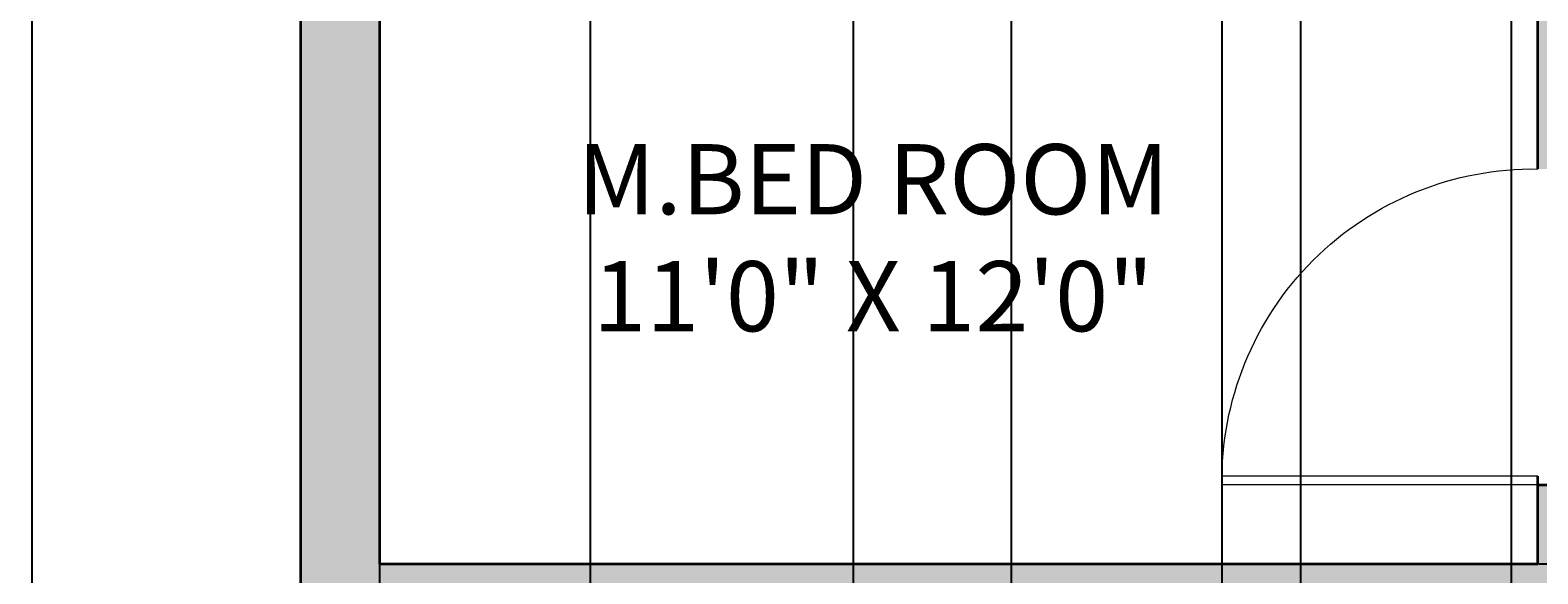
# Model space of a CAD drawing. Units: inches. Extents: x 1567 to 1964, y 1813 to 2447.
# Tile 13 of 28: x 1567 to 1738, y 2262 to 2324. Entities that reach past the tile are written whole.
import ezdxf

# ---------------------------------------------------------------- set-up
doc = ezdxf.new("R2010")
doc.units = ezdxf.units.IN
for name, color, linetype, lineweight in [('A-ANNO-DIMS', 2, 'Continuous', 18), ('A-AREA-IDEN', 7, 'Continuous', 18), ('A-DOOR', 4, 'Continuous', 18), ('A-WALL', 7, 'Continuous', 35)]:
    doc.layers.add(name, color=color, linetype=linetype, lineweight=lineweight)
doc.layers.add('A-WALL-PATT', color=251, linetype='Continuous', lineweight=13, true_color=0x636466)
doc.styles.get("Standard").update_dxf_attribs({"font": 'arial.ttf'})
doc.dimstyles.get("Standard").update_dxf_attribs({"dimtxt": 0.18, "dimasz": 0.18, "dimexe": 0.18, "dimexo": 0.0625, "dimgap": 0.09, "dimtad": 0, "dimtih": 1, "dimtoh": 1, "dimdec": 4, "dimzin": 0, "dimdsep": 46, "dimtxsty": 'Standard', "dimcen": 0.09, "dimadec": 0, "dimazin": 0, "dimtfac": 1, "dimtdec": 4, "dimtofl": 0, "dimtmove": 0, "dimatfit": 3, "dimfxl": 1, "dimtolj": 1, "dimtzin": 0, "dimarcsym": 0})

# ---------------------------------------------------------------- blocks, each defined once
blk = doc.blocks.new('DOOR-SWING-36IN')
for p, q in [((0, 36), (0, 0)), ((1, 36), (1, 0))]:
    blk.add_line(p, q)
blk.add_arc((0.5, 35.5), 35.5, 269.1931, 0.8069)
blk = doc.blocks.new('*D41')
at = {"layer": 'A-ANNO-DIMS', "color": 0, "lineweight": -2, "transparency": 16777216}
for p, q in [((1597.37, 2416.29), (1566.6, 2416.29)), ((1566.78, 2416.11), (1566.78, 2160.47)), ((1566.78, 1904.47), (1566.78, 2160.11)), ((1601.37, 1904.29), (1566.6, 1904.29))]:
    blk.add_line(p, q, dxfattribs=at)
at = {"layer": 'A-ANNO-DIMS', "color": 0, "transparency": 16777216}
for points in [[(1566.75, 2416.11), (1566.81, 2416.11), (1566.78, 2416.29)], [(1566.75, 1904.47), (1566.81, 1904.47), (1566.78, 1904.29)]]:
    blk.add_solid(points, dxfattribs=at)
at = {"layer": 'Defpoints', "color": 0, "transparency": 16777216}
for p in [(1566.78, 2416.29), (1597.43, 2416.29), (1601.43, 1904.29)]:
    blk.add_point(p, dxfattribs=at)
at = {"layer": 'A-ANNO-DIMS', "color": 0, "transparency": 16777216, "insert": (1566.78, 2160.29), "char_height": 0.18, "attachment_point": 5}
blk.add_mtext('\\A1;512', dxfattribs=at)
blk = doc.blocks.new('*D53')
at = {"layer": 'A-ANNO-DIMS', "color": 0, "lineweight": -2, "transparency": 16777216}
for p, q in [((1606.43, 1913.35), (1606.43, 2447.12)), ((1606.61, 2446.94), (1618.21, 2446.94)), ((1630.25, 2446.94), (1618.65, 2446.94)), ((1630.43, 1913.35), (1630.43, 2447.12))]:
    blk.add_line(p, q, dxfattribs=at)
at = {"layer": 'A-ANNO-DIMS', "color": 0, "transparency": 16777216}
for points in [[(1606.61, 2446.97), (1606.61, 2446.91), (1606.43, 2446.94)], [(1630.25, 2446.97), (1630.25, 2446.91), (1630.43, 2446.94)]]:
    blk.add_solid(points, dxfattribs=at)
at = {"layer": 'Defpoints', "color": 0, "transparency": 16777216}
for p in [(1630.43, 2446.94), (1606.43, 1913.29), (1630.43, 1913.29)]:
    blk.add_point(p, dxfattribs=at)
at = {"layer": 'A-ANNO-DIMS', "color": 0, "transparency": 16777216, "insert": (1618.43, 2446.94), "char_height": 0.18, "attachment_point": 5}
blk.add_mtext('\\A1;24', dxfattribs=at)
blk = doc.blocks.new('*D54')
at = {"layer": 'A-ANNO-DIMS', "color": 0, "lineweight": -2, "transparency": 16777216}
for p, q in [((1711.43, 1964.35), (1711.43, 2447.12)), ((1711.61, 2446.94), (1753.21, 2446.94)), ((1795.25, 2446.94), (1753.65, 2446.94)), ((1795.43, 1964.35), (1795.43, 2447.12))]:
    blk.add_line(p, q, dxfattribs=at)
at = {"layer": 'A-ANNO-DIMS', "color": 0, "transparency": 16777216}
for points in [[(1711.61, 2446.97), (1711.61, 2446.91), (1711.43, 2446.94)], [(1795.25, 2446.97), (1795.25, 2446.91), (1795.43, 2446.94)]]:
    blk.add_solid(points, dxfattribs=at)
at = {"layer": 'Defpoints', "color": 0, "transparency": 16777216}
for p in [(1795.43, 2446.94), (1711.43, 1964.29), (1795.43, 1964.29)]:
    blk.add_point(p, dxfattribs=at)
at = {"layer": 'A-ANNO-DIMS', "color": 0, "transparency": 16777216, "insert": (1753.43, 2446.94), "char_height": 0.18, "attachment_point": 5}
blk.add_mtext('\\A1;84', dxfattribs=at)
blk = doc.blocks.new('*D56')
at = {"layer": 'A-ANNO-DIMS', "color": 0, "lineweight": -2, "transparency": 16777216}
for p, q in [((1606.43, 2127.35), (1606.43, 2447.12)), ((1606.61, 2446.94), (1618.21, 2446.94)), ((1630.25, 2446.94), (1618.65, 2446.94)), ((1630.43, 2127.35), (1630.43, 2447.12))]:
    blk.add_line(p, q, dxfattribs=at)
at = {"layer": 'A-ANNO-DIMS', "color": 0, "transparency": 16777216}
for points in [[(1606.61, 2446.97), (1606.61, 2446.91), (1606.43, 2446.94)], [(1630.25, 2446.97), (1630.25, 2446.91), (1630.43, 2446.94)]]:
    blk.add_solid(points, dxfattribs=at)
at = {"layer": 'Defpoints', "color": 0, "transparency": 16777216}
for p in [(1630.43, 2446.94), (1606.43, 2127.29), (1630.43, 2127.29)]:
    blk.add_point(p, dxfattribs=at)
at = {"layer": 'A-ANNO-DIMS', "color": 0, "transparency": 16777216, "insert": (1618.43, 2446.94), "char_height": 0.18, "attachment_point": 5}
blk.add_mtext('\\A1;24', dxfattribs=at)
blk = doc.blocks.new('*D57')
at = {"layer": 'A-ANNO-DIMS', "color": 0, "lineweight": -2, "transparency": 16777216}
for p, q in [((1630.43, 2127.35), (1630.43, 2447.12)), ((1630.61, 2446.94), (1654.21, 2446.94)), ((1678.25, 2446.94), (1654.65, 2446.94)), ((1678.43, 2127.35), (1678.43, 2447.12))]:
    blk.add_line(p, q, dxfattribs=at)
at = {"layer": 'A-ANNO-DIMS', "color": 0, "transparency": 16777216}
for points in [[(1630.61, 2446.97), (1630.61, 2446.91), (1630.43, 2446.94)], [(1678.25, 2446.97), (1678.25, 2446.91), (1678.43, 2446.94)]]:
    blk.add_solid(points, dxfattribs=at)
at = {"layer": 'Defpoints', "color": 0, "transparency": 16777216}
for p in [(1678.43, 2446.94), (1630.43, 2127.29), (1678.43, 2127.29)]:
    blk.add_point(p, dxfattribs=at)
at = {"layer": 'A-ANNO-DIMS', "color": 0, "transparency": 16777216, "insert": (1654.43, 2446.94), "char_height": 0.18, "attachment_point": 5}
blk.add_mtext('\\A1;48', dxfattribs=at)
blk = doc.blocks.new('*D60')
at = {"layer": 'A-ANNO-DIMS', "color": 0, "lineweight": -2, "transparency": 16777216}
for p, q in [((1660.43, 2063.35), (1660.43, 2447.12)), ((1660.61, 2446.94), (1681.21, 2446.94)), ((1702.25, 2446.94), (1681.65, 2446.94)), ((1702.43, 2063.35), (1702.43, 2447.12))]:
    blk.add_line(p, q, dxfattribs=at)
at = {"layer": 'A-ANNO-DIMS', "color": 0, "transparency": 16777216}
for points in [[(1660.61, 2446.97), (1660.61, 2446.91), (1660.43, 2446.94)], [(1702.25, 2446.97), (1702.25, 2446.91), (1702.43, 2446.94)]]:
    blk.add_solid(points, dxfattribs=at)
at = {"layer": 'Defpoints', "color": 0, "transparency": 16777216}
for p in [(1660.43, 2446.94), (1660.43, 2063.29), (1702.43, 2063.29)]:
    blk.add_point(p, dxfattribs=at)
at = {"layer": 'A-ANNO-DIMS', "color": 0, "transparency": 16777216, "insert": (1681.43, 2446.94), "char_height": 0.18, "attachment_point": 5}
blk.add_mtext('\\A1;42', dxfattribs=at)
blk = doc.blocks.new('*D63')
at = {"layer": 'A-ANNO-DIMS', "color": 0, "lineweight": -2, "transparency": 16777216}
for p, q in [((1735.43, 1988.35), (1735.43, 2447.12)), ((1735.61, 2446.94), (1753.21, 2446.94)), ((1771.25, 2446.94), (1753.65, 2446.94)), ((1771.43, 1988.35), (1771.43, 2447.12))]:
    blk.add_line(p, q, dxfattribs=at)
at = {"layer": 'A-ANNO-DIMS', "color": 0, "transparency": 16777216}
for points in [[(1735.61, 2446.97), (1735.61, 2446.91), (1735.43, 2446.94)], [(1771.25, 2446.97), (1771.25, 2446.91), (1771.43, 2446.94)]]:
    blk.add_solid(points, dxfattribs=at)
at = {"layer": 'Defpoints', "color": 0, "transparency": 16777216}
for p in [(1771.43, 2446.94), (1735.43, 1988.29), (1771.43, 1988.29)]:
    blk.add_point(p, dxfattribs=at)
at = {"layer": 'A-ANNO-DIMS', "color": 0, "transparency": 16777216, "insert": (1753.43, 2446.94), "char_height": 0.18, "attachment_point": 5}
blk.add_mtext('\\A1;36', dxfattribs=at)
blk = doc.blocks.new('*D64')
at = {"layer": 'A-ANNO-DIMS', "color": 0, "lineweight": -2, "transparency": 16777216}
for p, q in [((1711.43, 2055.85), (1711.43, 2447.12)), ((1711.61, 2446.94), (1723.21, 2446.94)), ((1735.25, 2446.94), (1723.65, 2446.94)), ((1735.43, 2055.85), (1735.43, 2447.12))]:
    blk.add_line(p, q, dxfattribs=at)
at = {"layer": 'A-ANNO-DIMS', "color": 0, "transparency": 16777216}
for points in [[(1711.61, 2446.97), (1711.61, 2446.91), (1711.43, 2446.94)], [(1735.25, 2446.97), (1735.25, 2446.91), (1735.43, 2446.94)]]:
    blk.add_solid(points, dxfattribs=at)
at = {"layer": 'Defpoints', "color": 0, "transparency": 16777216}
for p in [(1735.43, 2446.94), (1711.43, 2055.79), (1735.43, 2055.79)]:
    blk.add_point(p, dxfattribs=at)
at = {"layer": 'A-ANNO-DIMS', "color": 0, "transparency": 16777216, "insert": (1723.43, 2446.94), "char_height": 0.18, "attachment_point": 5}
blk.add_mtext('\\A1;24', dxfattribs=at)
blk = doc.blocks.new('*D68')
at = {"layer": 'A-ANNO-DIMS', "color": 0, "lineweight": -2, "transparency": 16777216}
for p, q in [((1738.49, 2272.29), (1769.26, 2272.29)), ((1769.08, 2272.11), (1769.08, 2267.97)), ((1769.08, 2263.47), (1769.08, 2267.61)), ((1738.49, 2263.29), (1769.26, 2263.29))]:
    blk.add_line(p, q, dxfattribs=at)
at = {"layer": 'A-ANNO-DIMS', "color": 0, "transparency": 16777216}
for points in [[(1769.05, 2272.11), (1769.11, 2272.11), (1769.08, 2272.29)], [(1769.05, 2263.47), (1769.11, 2263.47), (1769.08, 2263.29)]]:
    blk.add_solid(points, dxfattribs=at)
at = {"layer": 'Defpoints', "color": 0, "transparency": 16777216}
for p in [(1738.43, 2272.29), (1738.43, 2263.29), (1769.08, 2263.29)]:
    blk.add_point(p, dxfattribs=at)
at = {"layer": 'A-ANNO-DIMS', "color": 0, "transparency": 16777216, "insert": (1769.08, 2267.79), "char_height": 0.18, "attachment_point": 5}
blk.add_mtext('\\A1;9', dxfattribs=at)

msp = doc.modelspace()

# ---------------------------------------------------------------- hatches: boundary and pattern name
at = {"layer": 'A-WALL-PATT'}
h = msp.add_hatch(color=256, dxfattribs=at)
h.dxf.hatch_style = 1
h.paths.add_polyline_path([(1606.4295, 2407.29), (1654.4295, 2407.29), (1654.4295, 2416.29), (1597.4295, 2416.29), (1597.4295, 2217.29), (1606.4295, 2217.29), (1606.4295, 2259.29), (1738.4295, 2259.29), (1738.4295, 2247.29), (1742.4295, 2247.29), (1742.4295, 2259.29), (1742.4295, 2272.29), (1738.4295, 2272.29), (1738.4295, 2263.29), (1606.4295, 2263.29)])
h.paths.add_polyline_path([(1753.4295, 2416.29), (1690.4295, 2416.29), (1690.4295, 2407.29), (1738.4295, 2407.29), (1738.4295, 2308.29), (1742.4295, 2308.29), (1742.4295, 2331.29), (1746.9295, 2331.29), (1746.9295, 2335.29), (1742.4295, 2335.29), (1742.4295, 2407.29), (1753.4295, 2407.29)])
h.paths.add_polyline_path([(1840.4295, 2416.29), (1777.4295, 2416.29), (1777.4295, 2407.29), (1788.4295, 2407.29), (1788.4295, 2335.29), (1776.9295, 2335.29), (1776.9295, 2331.29), (1788.4295, 2331.29), (1788.4295, 2308.29), (1792.4295, 2308.29), (1792.4295, 2407.29), (1840.4295, 2407.29)])
h.paths.add_polyline_path([(1933.4295, 2416.29), (1876.4295, 2416.29), (1876.4295, 2407.29), (1924.4295, 2407.29), (1924.4295, 2263.29), (1792.4295, 2263.29), (1792.4295, 2272.29), (1788.4295, 2272.29), (1788.4295, 2259.29), (1872.4295, 2259.29), (1872.4295, 2171.29), (1880.9295, 2171.29), (1880.9295, 2175.29), (1876.4295, 2175.29), (1876.4295, 2259.29), (1924.4295, 2259.29), (1924.4295, 2229.29), (1933.4295, 2229.29)])
h.paths.add_polyline_path([(1933.4295, 2205.29), (1924.4295, 2205.29), (1924.4295, 2175.29), (1910.9295, 2175.29), (1910.9295, 2171.29), (1924.4295, 2171.29), (1924.4295, 2127.29), (1844.4295, 2127.29), (1844.4295, 2123.29), (1924.4295, 2123.29), (1924.4295, 2063.29), (1933.4295, 2063.29)])
h.paths.add_polyline_path([(1799.4295, 2123.29), (1808.4295, 2123.29), (1808.4295, 2127.29), (1781.4295, 2127.29), (1781.4295, 2123.29), (1795.4295, 2123.29), (1795.4295, 1964.29), (1711.4295, 1964.29), (1711.4295, 2123.29), (1751.4295, 2123.29), (1751.4295, 2127.29), (1742.4295, 2127.29), (1742.4295, 2139.29), (1738.4295, 2139.29), (1738.4295, 2127.29), (1678.4295, 2127.29), (1678.4295, 2123.29), (1702.4295, 2123.29), (1702.4295, 1913.29), (1678.4295, 1913.29), (1678.4295, 1904.29), (1711.4295, 1904.29), (1711.4295, 1960.29), (1795.4295, 1960.29), (1795.4295, 1906.69), (1929.4295, 1906.69), (1929.4295, 1848.29), (1601.4295, 1848.29), (1601.4295, 1904.29), (1630.4295, 1904.29), (1630.4295, 1913.29), (1606.4295, 1913.29), (1606.4295, 2123.29), (1630.4295, 2123.29), (1630.4295, 2127.29), (1606.4295, 2127.29), (1606.4295, 2169.29), (1597.4295, 2169.29), (1597.4295, 1844.29), (1933.4295, 1844.29), (1933.4295, 2027.29), (1924.4295, 2027.29), (1924.4295, 1967.29), (1833.9295, 1967.29), (1833.9295, 1963.29), (1924.4295, 1963.29), (1924.4295, 1910.69), (1799.4295, 1910.69), (1799.4295, 1963.29), (1803.9295, 1963.29), (1803.9295, 1967.29), (1799.4295, 1967.29)])

# ---------------------------------------------------------------- linework, layer by layer
at = {"layer": 'A-WALL'}
for p, q in [((1597.4295, 1844.29), (1597.4295, 2416.29)), ((1606.4295, 2263.29), (1606.4295, 2407.29)), ((1738.4295, 2308.29), (1738.4295, 2407.29)), ((1738.4295, 2263.29), (1738.4295, 2273.29)), ((1738.4295, 2272.29), (1742.4295, 2272.29)), ((1606.4295, 2263.29), (1738.4295, 2263.29))]:
    msp.add_line(p, q, dxfattribs=at)

# ---------------------------------------------------------------- block references
at = {"layer": 'A-DOOR', "extrusion": (0, 0, -1), "zscale": -1, "rotation": 90.00000000011018}
msp.add_blockref('DOOR-SWING-36IN', (-1702.4285, 2272.2905), dxfattribs=at)

# ---------------------------------------------------------------- texts
at = {"layer": 'A-AREA-IDEN', "insert": (1621.8017, 2311.121), "char_height": 8, "attachment_point": 1}
msp.add_mtext_dynamic_manual_height_columns('\\pxqc;M.BED ROOM\\P11\'0" X 12\'0"', width=81.753814, gutter_width=12.5, heights=[0], dxfattribs=at)

# ---------------------------------------------------------------- dimensions: what is measured, and where the dimension line sits
at = {"layer": 'A-ANNO-DIMS'}
for base, p1, p2, picture, middle in [((1630.4295, 2446.94), (1606.4295, 1913.29), (1630.4295, 1913.29), '*D53', (1618.4295, 2446.94)), ((1630.4295, 2446.94), (1606.4295, 2127.29), (1630.4295, 2127.29), '*D56', (1618.4295, 2446.94)), ((1678.4295, 2446.94), (1630.4295, 2127.29), (1678.4295, 2127.29), '*D57', (1654.4295, 2446.94)), ((1660.4295, 2446.94), (1702.4295, 2063.29), (1660.4295, 2063.29), '*D60', (1681.4295, 2446.94)), ((1795.4295, 2446.94), (1711.4295, 1964.29), (1795.4295, 1964.29), '*D54', (1753.4295, 2446.94)), ((1735.4295, 2446.94), (1711.4295, 2055.79), (1735.4295, 2055.79), '*D64', (1723.4295, 2446.94)), ((1771.4295, 2446.94), (1735.4295, 1988.29), (1771.4295, 1988.29), '*D63', (1753.4295, 2446.94))]:
    dim = msp.add_linear_dim(base=base, p1=p1, p2=p2, dimstyle='Standard', override={"dimdec": 0, "dimlfac": 1, "dimrnd": 0, "dimzin": 0, "dimdsep": 46, "dimlunit": 2}, dxfattribs=at)
    dim.commit()
    dim.dimension.update_dxf_attribs({"geometry": picture, "text_midpoint": middle})
for base, p1, p2, angle, picture, middle in [((1566.7795, 2416.29), (1601.4295, 1904.29), (1597.4295, 2416.29), 90, '*D41', (1566.7795, 2160.29)), ((1769.0795, 2263.29), (1738.4295, 2272.29), (1738.4295, 2263.29), 270, '*D68', (1769.0795, 2267.79))]:
    dim = msp.add_linear_dim(base=base, p1=p1, p2=p2, angle=angle, dimstyle='Standard', override={"dimdec": 0, "dimlfac": 1, "dimrnd": 0, "dimzin": 0, "dimdsep": 46, "dimlunit": 2}, dxfattribs=at)
    dim.commit()
    dim.dimension.update_dxf_attribs({"geometry": picture, "text_midpoint": middle})

doc.saveas('drawing.dxf')
